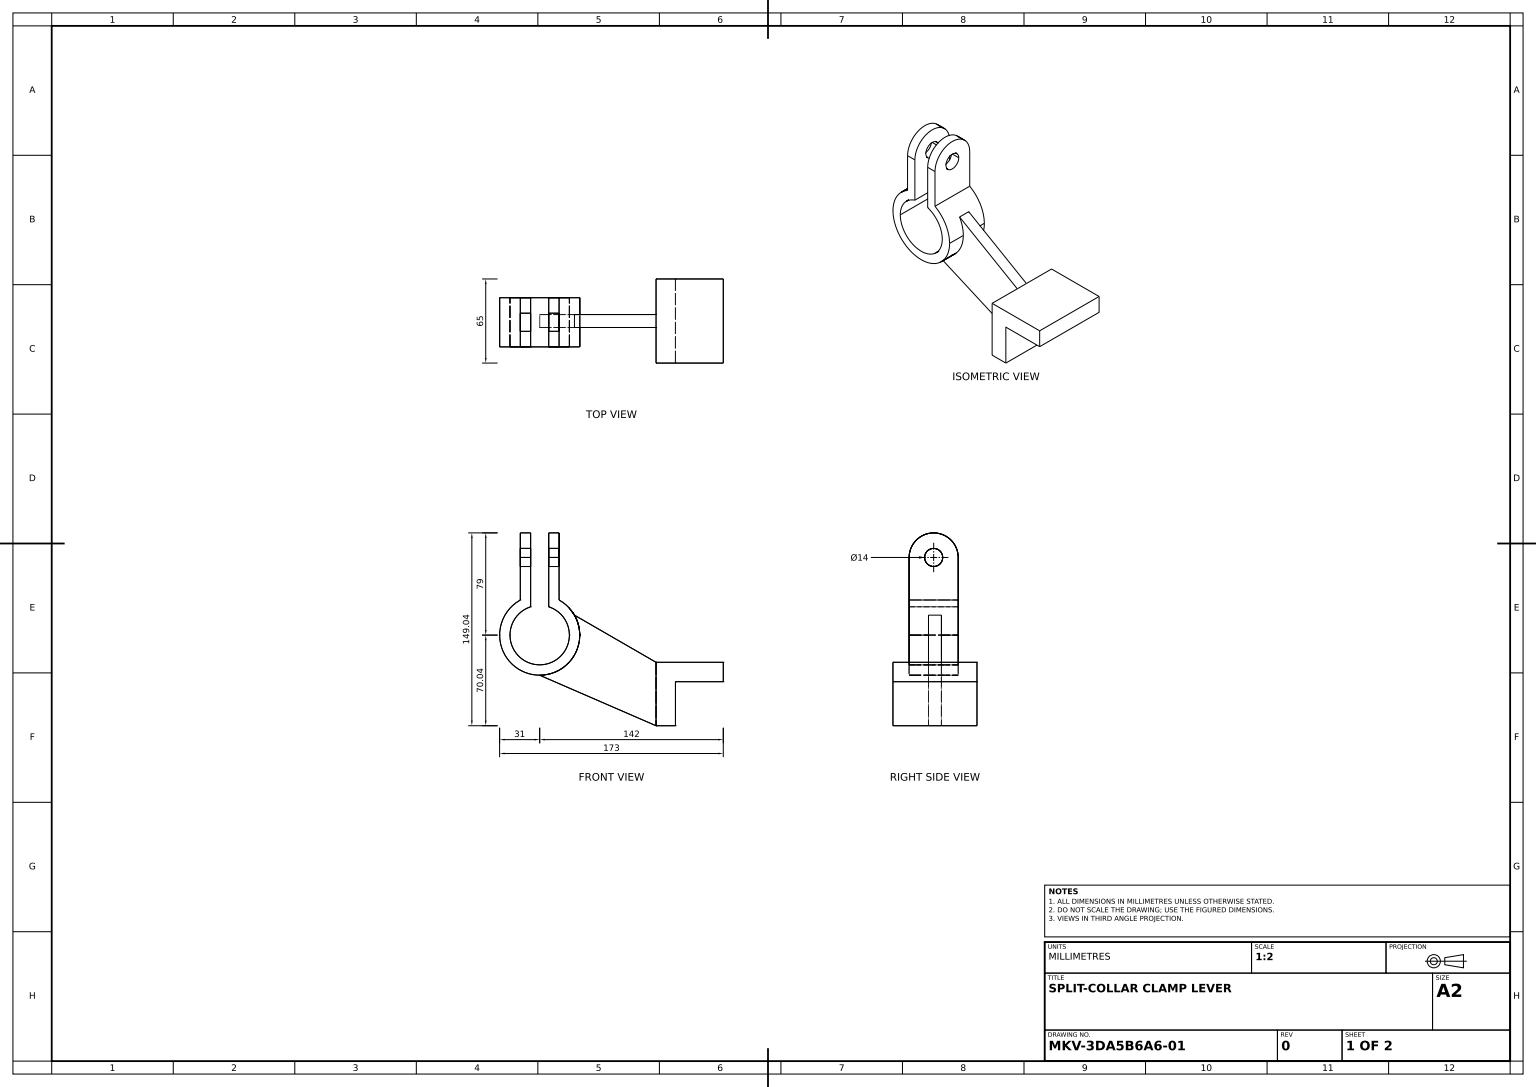
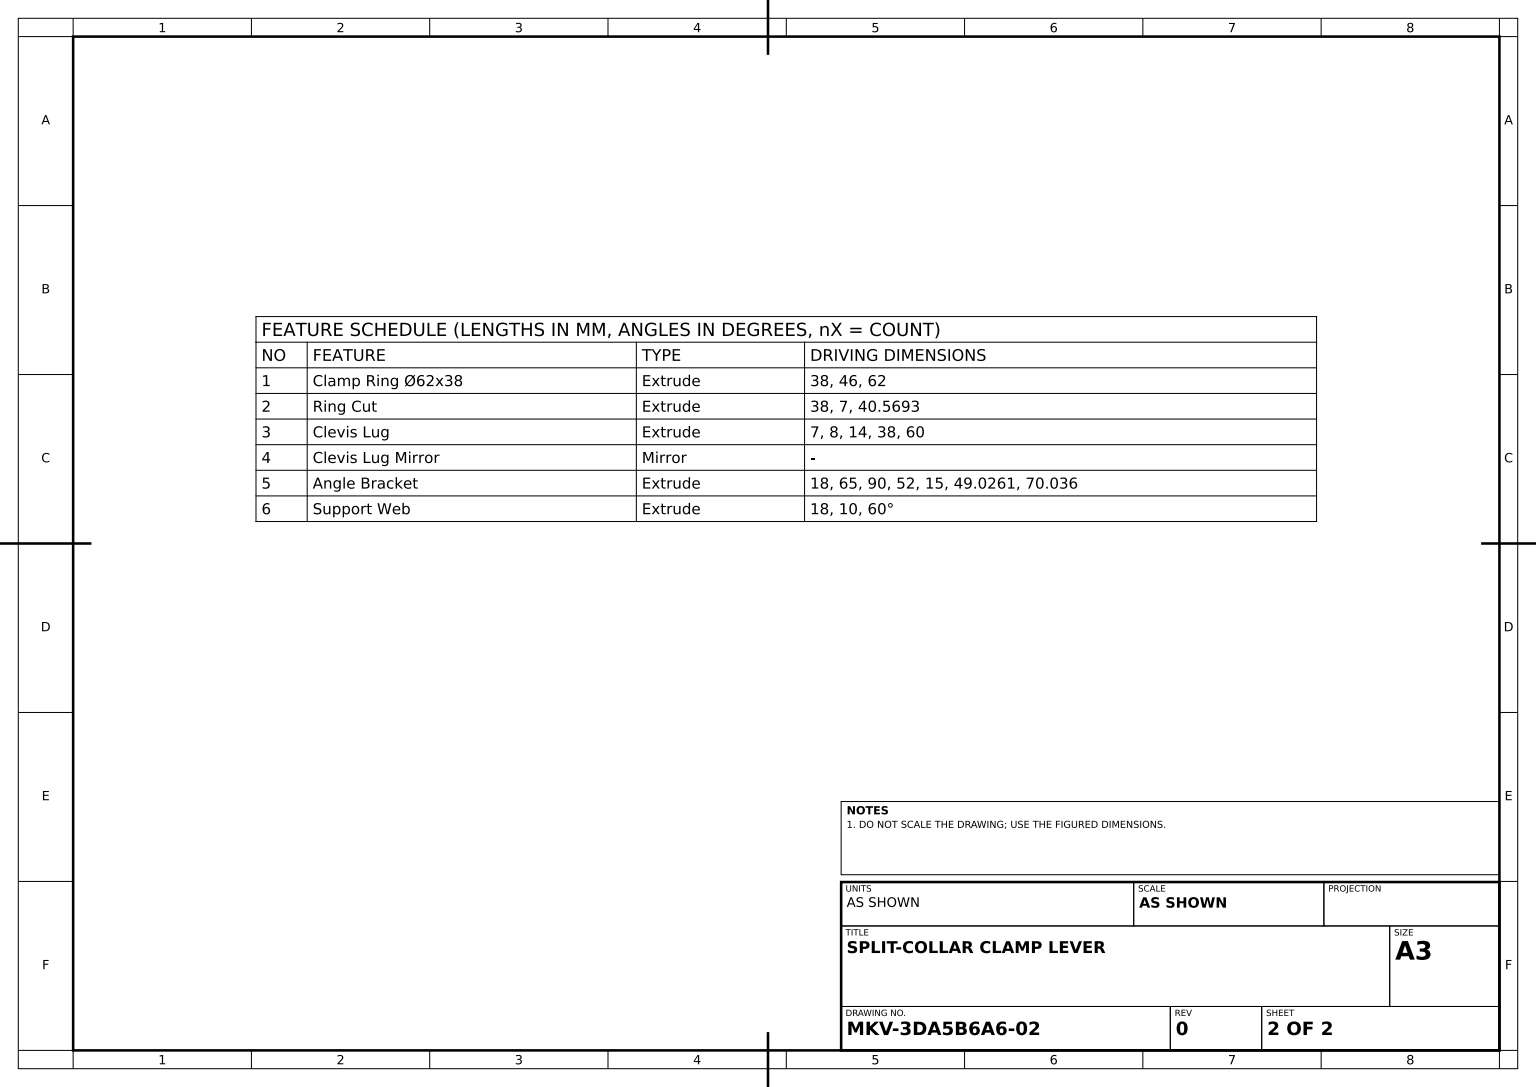
SolidWorks part; units mm, degrees
material "Plain Carbon Steel"
ref_plane "Front Plane" through (0, 0, 0) normal (0, 0, 1) x (1, 0, 0)
ref_plane "Top Plane" through (0, 0, 0) normal (0, 1, 0) x (1, 0, 0)
ref_plane "Right Plane" through (0, 0, 0) normal (1, 0, 0) x (0, 0, -1)
sketch "Clamp Ring Sketch Ø46-Ø62" plane through (0, 0, 0) normal (0, 0, 1) x (1, 0, 0)
  circle A0 centre (0, 0) radius 23
  circle A1 centre (0, 0) radius 31
  dimension "D1" = 46
  dimension "D2" = 62
extrude "Clamp Ring Ø62x38" add sketch "Clamp Ring Sketch Ø46-Ø62" along normal blind 38
ref_plane "Plane1" through (0, 0, 38) normal (0, 0, 1) x (1, 0, 0)
sketch "Ring Cut Sketch" plane through (0, 0, 38) normal (0, 0, 1) x (1, 0, 0)
  line L0 (0, 0) -> (0, 31) construction
  line L1 (0, 0) -> (-7, 0)
  line L2 (-7, 0) -> (-7, 40.5693)
  line L3 (0, 0) -> (7, 0)
  line L4 (7, 0) -> (7, 40.5693)
  line L5 (-7, 40.5693) -> (7, 40.5693)
  circle A0 centre (0, 0) radius 31 construction
  dimension "D1" = 7
  dimension "D2" = 40.5693
extrude "Ring Cut" cut sketch "Ring Cut Sketch" against normal blind 38
ref_plane "Plane2" through (7, 0, 0) normal (1, 0, 0) x (0, 0, -1)
sketch "Clevis Lug Sketch" plane through (7, 0, 0) normal (1, 0, 0) x (0, 0, -1)
  line L0 (-38, 60) -> (-38, 21.9089)
  line L1 (-38, 21.9089) -> (0, 21.9089)
  line L2 (0, -31) -> (0, 30.1993) construction
  line L3 (0, 21.9089) -> (0, 60)
  circle A0 centre (-19, 60) radius 7
  arc A1 (0, 60) -> (-38, 60) centre (-19, 60) ccw
  dimension "D1" = 14
  dimension "D2" = 38
  dimension "D3" = 60
extrude "Clevis Lug" add sketch "Clevis Lug Sketch" along normal blind 8
ref_plane "Plane3" through (0, 0, 0) normal (1, 0, 0) x (0, 0, -1)
mirror "Clevis Lug Mirror" about plane through (0, 0, 0) normal (1, 0, 0) of "Clevis Lug"
ref_plane "Plane4" through (0, 0, 18) normal (0, 0, 1) x (1, 0, 0)
sketch "Angle Bracket Sketch" plane through (0, 0, 18) normal (0, 0, 1) x (1, 0, 0)
  line L0 (90, -70.036) -> (105, -70.036)
  line L1 (90, -70.036) -> (90, -21.0099)
  line L2 (90, -21.0099) -> (142, -21.0099)
  line L3 (142, -21.0099) -> (142, -36.0099)
  line L4 (142, -36.0099) -> (105, -36.0099)
  line L5 (105, -36.0099) -> (105, -70.036)
  line L6 (90, -21.0099) -> (90, 57.8708) construction
  dimension "D1" = 90
  dimension "D2" = 52
  dimension "D3" = 15
  dimension "D4" = 15
  dimension "D5" = 49.0261
  dimension "D6" = 70.036
extrude "Angle Bracket" add sketch "Angle Bracket Sketch" along normal mid plane 65 separate body
sketch "Support Web Sketch 60deg" plane through (0, 0, 18) normal (0, 0, 1) x (1, 0, 0)
  line L0 (90, -70.036) -> (0, -31)
  line L1 (90, -21.0099) -> (90, 15.4018) construction
  line L2 (90, -21.0099) -> (26.8885, 15.4275)
  line L9 (90, -21.0099) -> (90, -70.036)
  line L10 (90, -70.036) -> (105, -70.036)
  line L11 (105, -70.036) -> (105, -36.0099)
  line L12 (105, -36.0099) -> (142, -36.0099)
  line L13 (142, -36.0099) -> (142, -21.0099)
  line L14 (142, -21.0099) -> (90, -21.0099)
  line L16 (90, -70.036) -> (105, -70.036)
  line L17 (105, -70.036) -> (105, -36.0099)
  line L18 (105, -36.0099) -> (142, -36.0099)
  line L19 (142, -36.0099) -> (142, -21.0099)
  line L20 (142, -21.0099) -> (90, -21.0099)
  arc A0 (-15, 27.1293) -> (15, 27.1293) centre (0, 0) ccw construction
  arc A1 (26.8885, 15.4275) -> (0, -31) centre (0, 0) cw
  dimension "D2" = 0
  dimension "D1" = 60
extrude "Support Web" add sketch "Support Web Sketch 60deg" along normal mid plane 10
